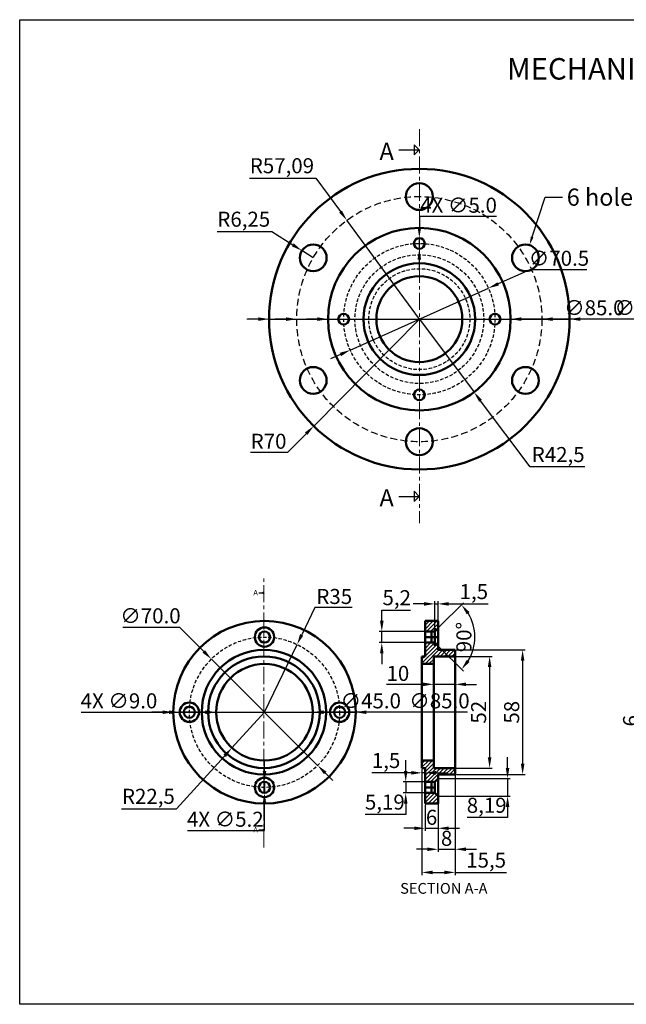
# Model space of a CAD drawing. Units: millimetres. Extents: x -42 to 606, y -195 to 264.
# Tile 1 of 3: x -42 to 240, y -195 to 264. Entities that reach past the tile are written whole.
import ezdxf
from ezdxf import colors
from ezdxf.entities.mleader import LeaderData, LeaderLine
from ezdxf.math import Vec2, Vec3

# ---------------------------------------------------------------- set-up
doc = ezdxf.new("R2010")
doc.units = ezdxf.units.MM
doc.header["$LTSCALE"] = 0.5
doc.linetypes.add('CENTER', pattern=[50.8, 31.75, -6.35, 6.35, -6.35])
doc.linetypes.add('HIDDEN', pattern=[9.525, 6.35, -3.175])
for name, color, linetype, lineweight in [('M-CNTR', 1, 'CENTER', 18), ('M-DIMS', 2, 'Continuous', 25), ('M-HATC', 8, 'Continuous', 18), ('M-HIDN', 4, 'HIDDEN', 25), ('M-OUTL', 7, 'Continuous', 50), ('M-SYMB', 3, 'Continuous', 25), ('M-TEXT', 3, 'Continuous', 25), ('M-TTLB', 7, 'Continuous', 25)]:
    doc.layers.add(name, color=color, linetype=linetype, lineweight=lineweight)
doc.styles.get("Standard").update_dxf_attribs({"font": 'arial.ttf'})
doc.dimstyles.new('ISO-25', dxfattribs={"dimtxt": 7, "dimasz": 5, "dimexe": 1.25, "dimexo": 0.625, "dimtad": 1, "dimtoh": 1, "dimtxsty": 'Standard', "dimcen": 2.5, "dimadec": 0, "dimazin": 0, "dimtfac": 1, "dimtmove": 0, "dimatfit": 3, "dimfxl": 1, "dimarcsym": 0})

# ---------------------------------------------------------------- blocks, each defined once
blk = doc.blocks.new('*D18')
at = {"layer": 'Defpoints', "color": 0, "ltscale": 0.5, "transparency": 16777216}
for p in [(88.97, 156.13), (94.25, 152.78)]:
    blk.add_point(p, dxfattribs=at)
at = {"layer": 'M-DIMS', "color": 0, "lineweight": -2, "ltscale": 0.5, "transparency": 16777216}
for p, q in [((49.45, 165.02), (75.01, 165.02)), ((75.01, 165.02), (84.76, 158.82)), ((94.25, 152.78), (88.97, 156.13))]:
    blk.add_line(p, q, dxfattribs=at)
at = {"layer": 'M-DIMS', "color": 0, "ltscale": 0.5, "transparency": 16777216}
blk.add_solid([(85.2, 159.52), (84.31, 158.11), (88.97, 156.13)], dxfattribs=at)
at = {"layer": 'M-DIMS', "color": 0, "ltscale": 0.5, "transparency": 16777216, "insert": (61.91, 169.85), "char_height": 7, "attachment_point": 5}
blk.add_mtext('R6,25', dxfattribs=at)
blk = doc.blocks.new('*D19')
at = {"layer": 'Defpoints', "color": 0, "ltscale": 0.5, "transparency": 16777216}
for p in [(143.69, 124.23), (94.49, 74.44)]:
    blk.add_point(p, dxfattribs=at)
at = {"layer": 'M-DIMS', "color": 0, "lineweight": -2, "ltscale": 0.5, "transparency": 16777216}
for p, q in [((143.69, 124.23), (94.49, 74.44)), ((82.43, 62.24), (90.97, 70.88)), ((65.11, 62.24), (82.43, 62.24))]:
    blk.add_line(p, q, dxfattribs=at)
at = {"layer": 'M-DIMS', "color": 0, "ltscale": 0.5, "transparency": 16777216}
blk.add_solid([(90.38, 71.47), (91.56, 70.3), (94.49, 74.44)], dxfattribs=at)
at = {"layer": 'M-DIMS', "color": 0, "ltscale": 0.5, "transparency": 16777216, "insert": (73.46, 66.44), "char_height": 7, "attachment_point": 5}
blk.add_mtext('R70', dxfattribs=at)
blk = doc.blocks.new('*D20')
at = {"layer": 'Defpoints', "color": 0, "ltscale": 0.5, "transparency": 16777216}
for p in [(143.69, 124.23), (169.18, 90.22)]:
    blk.add_point(p, dxfattribs=at)
at = {"layer": 'M-DIMS', "color": 0, "lineweight": -2, "ltscale": 0.5, "transparency": 16777216}
for p, q in [((143.69, 124.23), (169.18, 90.22)), ((195.26, 55.43), (172.18, 86.22)), ((220.82, 55.43), (195.26, 55.43))]:
    blk.add_line(p, q, dxfattribs=at)
at = {"layer": 'M-DIMS', "color": 0, "ltscale": 0.5, "transparency": 16777216}
blk.add_solid([(172.85, 86.72), (171.51, 85.72), (169.18, 90.22)], dxfattribs=at)
at = {"layer": 'M-DIMS', "color": 0, "ltscale": 0.5, "transparency": 16777216, "insert": (208.36, 60.26), "char_height": 7, "attachment_point": 5}
blk.add_mtext('R42,5', dxfattribs=at)
blk = doc.blocks.new('*D21')
at = {"layer": 'Defpoints', "color": 0, "ltscale": 0.5, "transparency": 16777216}
for p in [(109.92, 170.26), (143.69, 124.23)]:
    blk.add_point(p, dxfattribs=at)
at = {"layer": 'M-DIMS', "color": 0, "lineweight": -2, "ltscale": 0.5, "transparency": 16777216}
for p, q in [((64.53, 189.93), (95.49, 189.93)), ((95.49, 189.93), (106.96, 174.29)), ((143.69, 124.23), (109.92, 170.26))]:
    blk.add_line(p, q, dxfattribs=at)
at = {"layer": 'M-DIMS', "color": 0, "ltscale": 0.5, "transparency": 16777216}
blk.add_solid([(107.63, 174.78), (106.29, 173.8), (109.92, 170.26)], dxfattribs=at)
at = {"layer": 'M-DIMS', "color": 0, "ltscale": 0.5, "transparency": 16777216, "insert": (79.69, 194.76), "char_height": 7, "attachment_point": 5}
blk.add_mtext('R57,09', dxfattribs=at)
blk = doc.blocks.new('*D23')
at = {"layer": 'Defpoints', "color": 0, "ltscale": 0.5, "transparency": 16777216}
for p in [(255.34, -59.83), (247.18, -65.83), (255.34, -65.83)]:
    blk.add_point(p, dxfattribs=at)
at = {"layer": 'M-DIMS', "color": 0, "lineweight": -2, "ltscale": 0.5, "transparency": 16777216}
for p, q in [((247.18, -54.83), (247.18, -49.83)), ((254.71, -59.83), (245.93, -59.83)), ((247.18, -59.83), (247.18, -65.83)), ((254.71, -65.83), (245.93, -65.83)), ((247.18, -70.83), (247.18, -75.83))]:
    blk.add_line(p, q, dxfattribs=at)
at = {"layer": 'M-DIMS', "color": 0, "ltscale": 0.5, "transparency": 16777216}
for points in [[(246.34, -54.83), (248.01, -54.83), (247.18, -59.83)], [(246.34, -70.83), (248.01, -70.83), (247.18, -65.83)]]:
    blk.add_solid(points, dxfattribs=at)
at = {"layer": 'M-DIMS', "color": 0, "ltscale": 0.5, "transparency": 16777216, "insert": (242.98, -62.83), "char_height": 7, "attachment_point": 5, "rotation": 90}
blk.add_mtext('6', dxfattribs=at)
blk = doc.blocks.new('*D51')
at = {"layer": 'Defpoints', "color": 0, "ltscale": 0.5, "transparency": 16777216}
for p in [(160.39, -32.83), (160.39, -84.83), (176.42, -84.83)]:
    blk.add_point(p, dxfattribs=at)
at = {"layer": 'M-DIMS', "color": 0, "lineweight": -2, "ltscale": 0.5, "transparency": 16777216}
for p, q in [((161.01, -32.83), (177.67, -32.83)), ((176.42, -37.83), (176.42, -79.83)), ((161.01, -84.83), (177.67, -84.83))]:
    blk.add_line(p, q, dxfattribs=at)
at = {"layer": 'M-DIMS', "color": 0, "ltscale": 0.5, "transparency": 16777216}
for points in [[(175.58, -37.83), (177.25, -37.83), (176.42, -32.83)], [(175.58, -79.83), (177.25, -79.83), (176.42, -84.83)]]:
    blk.add_solid(points, dxfattribs=at)
at = {"layer": 'M-DIMS', "color": 0, "ltscale": 0.5, "transparency": 16777216, "insert": (172.22, -58.83), "char_height": 7, "attachment_point": 5, "rotation": 90}
blk.add_mtext('52', dxfattribs=at)
blk = doc.blocks.new('*D52')
at = {"layer": 'Defpoints', "color": 0, "ltscale": 0.5, "transparency": 16777216}
for p in [(160.39, -29.83), (160.39, -87.83), (191.8, -87.83)]:
    blk.add_point(p, dxfattribs=at)
at = {"layer": 'M-DIMS', "color": 0, "lineweight": -2, "ltscale": 0.5, "transparency": 16777216}
for p, q in [((161.01, -29.83), (193.05, -29.83)), ((191.8, -34.83), (191.8, -82.83)), ((161.01, -87.83), (193.05, -87.83))]:
    blk.add_line(p, q, dxfattribs=at)
at = {"layer": 'M-DIMS', "color": 0, "ltscale": 0.5, "transparency": 16777216}
for points in [[(190.97, -34.83), (192.63, -34.83), (191.8, -29.83)], [(190.97, -82.83), (192.63, -82.83), (191.8, -87.83)]]:
    blk.add_solid(points, dxfattribs=at)
at = {"layer": 'M-DIMS', "color": 0, "ltscale": 0.5, "transparency": 16777216, "insert": (187.6, -58.83), "char_height": 7, "attachment_point": 5, "rotation": 90}
blk.add_mtext('58', dxfattribs=at)
blk = doc.blocks.new('*D53')
at = {"layer": 'Defpoints', "color": 0, "ltscale": 0.5, "transparency": 16777216}
for p in [(152.39, -8.38), (150.89, -19.73), (152.39, -19.73)]:
    blk.add_point(p, dxfattribs=at)
at = {"layer": 'M-DIMS', "color": 0, "lineweight": -2, "ltscale": 0.5, "transparency": 16777216}
for p, q in [((145.89, -8.38), (140.89, -8.38)), ((150.89, -19.1), (150.89, -7.13)), ((150.89, -8.38), (152.39, -8.38)), ((152.39, -19.1), (152.39, -7.13)), ((157.39, -8.38), (175.78, -8.38))]:
    blk.add_line(p, q, dxfattribs=at)
at = {"layer": 'M-DIMS', "color": 0, "ltscale": 0.5, "transparency": 16777216}
for points in [[(145.89, -7.55), (145.89, -9.22), (150.89, -8.38)], [(157.39, -7.55), (157.39, -9.22), (152.39, -8.38)]]:
    blk.add_solid(points, dxfattribs=at)
at = {"layer": 'M-DIMS', "color": 0, "ltscale": 0.5, "transparency": 16777216, "insert": (169.08, -3.55), "char_height": 7, "attachment_point": 5}
blk.add_mtext('1,5', dxfattribs=at)
blk = doc.blocks.new('*D54')
at = {"layer": 'Defpoints', "color": 0, "ltscale": 0.5, "transparency": 16777216}
for p in [(146.39, -21.23), (126.2, -26.43), (146.39, -26.43)]:
    blk.add_point(p, dxfattribs=at)
at = {"layer": 'M-DIMS', "color": 0, "lineweight": -2, "ltscale": 0.5, "transparency": 16777216}
for p, q in [((126.2, -16.23), (126.2, -11.23)), ((126.2, -11.23), (139.5, -11.23)), ((145.76, -21.23), (124.95, -21.23)), ((126.2, -26.43), (126.2, -21.23)), ((145.76, -26.43), (124.95, -26.43)), ((126.2, -31.43), (126.2, -36.43))]:
    blk.add_line(p, q, dxfattribs=at)
at = {"layer": 'M-DIMS', "color": 0, "ltscale": 0.5, "transparency": 16777216}
for points in [[(125.37, -16.23), (127.03, -16.23), (126.2, -21.23)], [(125.37, -31.43), (127.03, -31.43), (126.2, -26.43)]]:
    blk.add_solid(points, dxfattribs=at)
at = {"layer": 'M-DIMS', "color": 0, "ltscale": 0.5, "transparency": 16777216, "insert": (133.16, -6.39), "char_height": 7, "attachment_point": 5}
blk.add_mtext('5,2', dxfattribs=at)
blk = doc.blocks.new('*D55')
at = {"layer": 'Defpoints', "color": 0, "ltscale": 0.5, "transparency": 16777216}
for p in [(160.39, -45.84), (150.39, -46.83), (160.39, -46.83)]:
    blk.add_point(p, dxfattribs=at)
at = {"layer": 'M-DIMS', "color": 0, "lineweight": -2, "ltscale": 0.5, "transparency": 16777216}
for p, q in [((145.39, -45.84), (128.4, -45.84)), ((150.39, -46.2), (150.39, -44.59)), ((160.39, -45.84), (150.39, -45.84)), ((160.39, -46.2), (160.39, -44.59)), ((165.39, -45.84), (170.39, -45.84))]:
    blk.add_line(p, q, dxfattribs=at)
at = {"layer": 'M-DIMS', "color": 0, "ltscale": 0.5, "transparency": 16777216}
for points in [[(145.39, -45.01), (145.39, -46.67), (150.39, -45.84)], [(165.39, -45.01), (165.39, -46.67), (160.39, -45.84)]]:
    blk.add_solid(points, dxfattribs=at)
at = {"layer": 'M-DIMS', "color": 0, "ltscale": 0.5, "transparency": 16777216, "insert": (133.7, -41.64), "char_height": 7, "attachment_point": 5}
blk.add_mtext('10', dxfattribs=at)
blk = doc.blocks.new('*D56')
at = {"layer": 'Defpoints', "color": 0, "ltscale": 0.5, "transparency": 16777216}
for p in [(144.89, -84.83), (144.89, -87.05), (146.39, -84.83)]:
    blk.add_point(p, dxfattribs=at)
at = {"layer": 'M-DIMS', "color": 0, "lineweight": -2, "ltscale": 0.5, "transparency": 16777216}
for p, q in [((139.89, -87.05), (121.5, -87.05)), ((144.89, -85.45), (144.89, -88.3)), ((146.39, -87.05), (144.89, -87.05)), ((146.39, -85.45), (146.39, -88.3)), ((151.39, -87.05), (156.39, -87.05))]:
    blk.add_line(p, q, dxfattribs=at)
at = {"layer": 'M-DIMS', "color": 0, "ltscale": 0.5, "transparency": 16777216}
for points in [[(139.89, -86.22), (139.89, -87.89), (144.89, -87.05)], [(151.39, -86.22), (151.39, -87.89), (146.39, -87.05)]]:
    blk.add_solid(points, dxfattribs=at)
at = {"layer": 'M-DIMS', "color": 0, "ltscale": 0.5, "transparency": 16777216, "insert": (128.2, -82.22), "char_height": 7, "attachment_point": 5}
blk.add_mtext('1,5', dxfattribs=at)
blk = doc.blocks.new('*D57')
at = {"layer": 'Defpoints', "color": 0, "ltscale": 0.5, "transparency": 16777216}
for p in [(150.89, -21.24), (152.39, -19.74), (150.89, -26.43), (152.39, -27.93), (168.83, -29.33)]:
    blk.add_point(p, dxfattribs=at)
at = {"layer": 'M-DIMS', "color": 0, "lineweight": -2, "ltscale": 0.5, "transparency": 16777216}
for p, q in [((152.83, -19.29), (164.21, -7.91)), ((152.83, -28.37), (164.21, -39.75))]:
    blk.add_line(p, q, dxfattribs=at)
blk.add_arc((148.29, -23.83), 21.26, 328.507, 31.493, dxfattribs=at)
at = {"layer": 'M-DIMS', "color": 0, "ltscale": 0.5, "transparency": 16777216}
for points in [[(165.77, -13.24), (167.08, -12.21), (163.33, -8.8)], [(167.08, -35.45), (165.77, -34.42), (163.33, -38.86)]]:
    blk.add_solid(points, dxfattribs=at)
at = {"layer": 'M-DIMS', "color": 0, "ltscale": 0.5, "transparency": 16777216, "insert": (165.35, -23.83), "char_height": 7, "attachment_point": 5, "rotation": 90}
blk.add_mtext('90°', dxfattribs=at)
blk = doc.blocks.new('*D58')
at = {"layer": 'Defpoints', "color": 0, "ltscale": 0.5, "transparency": 16777216}
for p in [(146.39, -101.33), (152.39, -101.33), (152.39, -112.87)]:
    blk.add_point(p, dxfattribs=at)
at = {"layer": 'M-DIMS', "color": 0, "lineweight": -2, "ltscale": 0.5, "transparency": 16777216}
for p, q in [((146.39, -101.95), (146.39, -114.12)), ((152.39, -101.95), (152.39, -114.12)), ((141.39, -112.87), (136.39, -112.87)), ((146.39, -112.87), (152.39, -112.87)), ((157.39, -112.87), (162.39, -112.87))]:
    blk.add_line(p, q, dxfattribs=at)
at = {"layer": 'M-DIMS', "color": 0, "ltscale": 0.5, "transparency": 16777216}
for points in [[(141.39, -112.04), (141.39, -113.7), (146.39, -112.87)], [(157.39, -112.04), (157.39, -113.7), (152.39, -112.87)]]:
    blk.add_solid(points, dxfattribs=at)
at = {"layer": 'M-DIMS', "color": 0, "ltscale": 0.5, "transparency": 16777216, "insert": (149.39, -108.67), "char_height": 7, "attachment_point": 5}
blk.add_mtext('6', dxfattribs=at)
blk = doc.blocks.new('*D59')
at = {"layer": 'Defpoints', "color": 0, "ltscale": 0.5, "transparency": 16777216}
for p in [(152.39, -87.83), (160.39, -87.83), (160.39, -122.64)]:
    blk.add_point(p, dxfattribs=at)
at = {"layer": 'M-DIMS', "color": 0, "lineweight": -2, "ltscale": 0.5, "transparency": 16777216}
for p, q in [((152.39, -88.45), (152.39, -123.89)), ((160.39, -88.45), (160.39, -123.89)), ((147.39, -122.64), (142.39, -122.64)), ((152.39, -122.64), (160.39, -122.64)), ((165.39, -122.64), (170.39, -122.64))]:
    blk.add_line(p, q, dxfattribs=at)
at = {"layer": 'M-DIMS', "color": 0, "ltscale": 0.5, "transparency": 16777216}
for points in [[(147.39, -121.81), (147.39, -123.47), (152.39, -122.64)], [(165.39, -121.81), (165.39, -123.47), (160.39, -122.64)]]:
    blk.add_solid(points, dxfattribs=at)
at = {"layer": 'M-DIMS', "color": 0, "ltscale": 0.5, "transparency": 16777216, "insert": (156.39, -118.44), "char_height": 7, "attachment_point": 5}
blk.add_mtext('8', dxfattribs=at)
blk = doc.blocks.new('*D60')
at = {"layer": 'Defpoints', "color": 0, "ltscale": 0.5, "transparency": 16777216}
for p in [(144.89, -84.83), (160.39, -84.83), (160.39, -133.42)]:
    blk.add_point(p, dxfattribs=at)
at = {"layer": 'M-DIMS', "color": 0, "lineweight": -2, "ltscale": 0.5, "transparency": 16777216}
for p, q in [((144.89, -85.45), (144.89, -134.67)), ((160.39, -85.45), (160.39, -134.67)), ((149.89, -133.42), (155.39, -133.42)), ((160.39, -133.42), (184.22, -133.42))]:
    blk.add_line(p, q, dxfattribs=at)
at = {"layer": 'M-DIMS', "color": 0, "ltscale": 0.5, "transparency": 16777216}
for points in [[(149.89, -132.59), (149.89, -134.26), (144.89, -133.42)], [(155.39, -132.59), (155.39, -134.26), (160.39, -133.42)]]:
    blk.add_solid(points, dxfattribs=at)
at = {"layer": 'M-DIMS', "color": 0, "ltscale": 0.5, "transparency": 16777216, "insert": (174.8, -128.59), "char_height": 7, "attachment_point": 5}
blk.add_mtext('15,5', dxfattribs=at)
blk = doc.blocks.new('*D61')
at = {"layer": 'Defpoints', "color": 0, "ltscale": 0.5, "transparency": 16777216}
for p in [(146.39, -91.23), (137.35, -96.41), (146.39, -96.41)]:
    blk.add_point(p, dxfattribs=at)
at = {"layer": 'M-DIMS', "color": 0, "lineweight": -2, "ltscale": 0.5, "transparency": 16777216}
for p, q in [((137.35, -86.23), (137.35, -81.23)), ((145.76, -91.23), (136.1, -91.23)), ((137.35, -91.23), (137.35, -96.41)), ((145.76, -96.41), (136.1, -96.41)), ((137.35, -101.41), (137.35, -106.41)), ((137.35, -106.41), (118.53, -106.41))]:
    blk.add_line(p, q, dxfattribs=at)
at = {"layer": 'M-DIMS', "color": 0, "ltscale": 0.5, "transparency": 16777216}
for points in [[(136.51, -86.23), (138.18, -86.23), (137.35, -91.23)], [(136.51, -101.41), (138.18, -101.41), (137.35, -96.41)]]:
    blk.add_solid(points, dxfattribs=at)
at = {"layer": 'M-DIMS', "color": 0, "ltscale": 0.5, "transparency": 16777216, "insert": (127.62, -101.58), "char_height": 7, "attachment_point": 5}
blk.add_mtext('5,19', dxfattribs=at)
blk = doc.blocks.new('*D62')
at = {"layer": 'Defpoints', "color": 0, "ltscale": 0.5, "transparency": 16777216}
for p in [(152.39, -89.73), (152.39, -97.91), (184.79, -97.91)]:
    blk.add_point(p, dxfattribs=at)
at = {"layer": 'M-DIMS', "color": 0, "lineweight": -2, "ltscale": 0.5, "transparency": 16777216}
for p, q in [((184.79, -84.73), (184.79, -79.73)), ((153.01, -89.73), (186.04, -89.73)), ((184.79, -89.73), (184.79, -97.91)), ((153.01, -97.91), (186.04, -97.91)), ((184.79, -102.91), (184.79, -107.91)), ((184.79, -107.91), (165.96, -107.91))]:
    blk.add_line(p, q, dxfattribs=at)
at = {"layer": 'M-DIMS', "color": 0, "ltscale": 0.5, "transparency": 16777216}
for points in [[(183.95, -84.73), (185.62, -84.73), (184.79, -89.73)], [(183.95, -102.91), (185.62, -102.91), (184.79, -97.91)]]:
    blk.add_solid(points, dxfattribs=at)
at = {"layer": 'M-DIMS', "color": 0, "ltscale": 0.5, "transparency": 16777216, "insert": (175.06, -103.08), "char_height": 7, "attachment_point": 5}
blk.add_mtext('8,19', dxfattribs=at)
blk = doc.blocks.new('*D63')
at = {"layer": 'Defpoints', "color": 0, "ltscale": 0.5, "transparency": 16777216}
for p in [(71.56, -58.83), (56.39, -75.44)]:
    blk.add_point(p, dxfattribs=at)
at = {"layer": 'M-DIMS', "color": 0, "lineweight": -2, "ltscale": 0.5, "transparency": 16777216}
for p, q in [((71.56, -58.83), (56.39, -75.44)), ((30.57, -103.74), (53.02, -79.14)), ((5.01, -103.74), (30.57, -103.74))]:
    blk.add_line(p, q, dxfattribs=at)
at = {"layer": 'M-DIMS', "color": 0, "ltscale": 0.5, "transparency": 16777216}
blk.add_solid([(52.41, -78.58), (53.64, -79.7), (56.39, -75.44)], dxfattribs=at)
at = {"layer": 'M-DIMS', "color": 0, "ltscale": 0.5, "transparency": 16777216, "insert": (17.48, -98.9), "char_height": 7, "attachment_point": 5}
blk.add_mtext('R22,5', dxfattribs=at)
blk = doc.blocks.new('*D64')
at = {"layer": 'Defpoints', "color": 0, "ltscale": 0.5, "transparency": 16777216}
for p in [(86.74, -27.29), (71.56, -58.83)]:
    blk.add_point(p, dxfattribs=at)
at = {"layer": 'M-DIMS', "color": 0, "lineweight": -2, "ltscale": 0.5, "transparency": 16777216}
for p, q in [((95.04, -10.03), (88.9, -22.78)), ((112.44, -10.03), (95.04, -10.03)), ((71.56, -58.83), (86.74, -27.29))]:
    blk.add_line(p, q, dxfattribs=at)
at = {"layer": 'M-DIMS', "color": 0, "ltscale": 0.5, "transparency": 16777216}
blk.add_solid([(88.15, -22.42), (89.65, -23.14), (86.74, -27.29)], dxfattribs=at)
at = {"layer": 'M-DIMS', "color": 0, "ltscale": 0.5, "transparency": 16777216, "insert": (104.05, -5.83), "char_height": 7, "attachment_point": 5}
blk.add_mtext('R35', dxfattribs=at)
blk = doc.blocks.new('SECTION-ARROW')
at = {"ltscale": 0.5}
for p, q in [((0, 0.39), (2.47, 0.39)), ((2.47, 0.39), (2.07, 0.78)), ((2.07, 0.78), (2.07, 0)), ((2.47, 0.39), (2.07, 0))]:
    blk.add_line(p, q, dxfattribs=at)
blk = doc.blocks.new('SECTION-ARROW-LG')
at = {"ltscale": 0.5}
for p, q in [((9.52, 2.39), (7.13, 4.78)), ((7.13, 4.78), (7.13, 0)), ((0, 2.39), (9.52, 2.39)), ((9.52, 2.39), (7.13, 0))]:
    blk.add_line(p, q, dxfattribs=at)
blk = doc.blocks.new('*D68')
at = {"layer": 'Defpoints', "color": 0, "ltscale": 0.5, "transparency": 16777216}
for p in [(73.69, 124.23), (213.69, 124.23)]:
    blk.add_point(p, dxfattribs=at)
at = {"layer": 'M-DIMS', "color": 0, "lineweight": -2, "ltscale": 0.5, "transparency": 16777216}
for p, q in [((68.69, 124.23), (63.69, 124.23)), ((73.69, 124.23), (213.69, 124.23)), ((255.69, 124.23), (218.69, 124.23)), ((287.53, 124.23), (255.69, 124.23))]:
    blk.add_line(p, q, dxfattribs=at)
at = {"layer": 'M-DIMS', "color": 0, "ltscale": 0.5, "transparency": 16777216}
for points in [[(68.69, 125.06), (68.69, 123.4), (73.69, 124.23)], [(218.69, 125.06), (218.69, 123.4), (213.69, 124.23)]]:
    blk.add_solid(points, dxfattribs=at)
at = {"layer": 'M-DIMS', "color": 0, "ltscale": 0.5, "transparency": 16777216, "insert": (271.92, 128.62), "char_height": 7, "attachment_point": 5}
blk.add_mtext('∅140.0', dxfattribs=at)
blk = doc.blocks.new('*D69')
at = {"layer": 'Defpoints', "color": 0, "ltscale": 0.5, "transparency": 16777216}
for p in [(86.6, 124.23), (200.78, 124.23)]:
    blk.add_point(p, dxfattribs=at)
at = {"layer": 'M-DIMS', "color": 0, "lineweight": -2, "ltscale": 0.5, "transparency": 16777216}
for p, q in [((81.6, 124.23), (76.6, 124.23)), ((86.6, 124.23), (200.78, 124.23)), ((235.03, 124.23), (205.78, 124.23)), ((272.35, 124.23), (235.03, 124.23))]:
    blk.add_line(p, q, dxfattribs=at)
at = {"layer": 'M-DIMS', "color": 0, "ltscale": 0.5, "transparency": 16777216}
for points in [[(81.6, 125.06), (81.6, 123.4), (86.6, 124.23)], [(205.78, 125.06), (205.78, 123.4), (200.78, 124.23)]]:
    blk.add_solid(points, dxfattribs=at)
at = {"layer": 'M-DIMS', "color": 0, "ltscale": 0.5, "transparency": 16777216, "insert": (254, 128.62), "char_height": 7, "attachment_point": 5}
blk.add_mtext('∅114.18', dxfattribs=at)
blk = doc.blocks.new('*D70')
at = {"layer": 'Defpoints', "color": 0, "ltscale": 0.5, "transparency": 16777216}
for p in [(101.19, 124.23), (186.19, 124.23)]:
    blk.add_point(p, dxfattribs=at)
at = {"layer": 'M-DIMS', "color": 0, "lineweight": -2, "ltscale": 0.5, "transparency": 16777216}
for p, q in [((96.19, 124.23), (91.19, 124.23)), ((101.19, 124.23), (186.19, 124.23)), ((211.69, 124.23), (191.19, 124.23)), ((238.09, 124.23), (211.69, 124.23))]:
    blk.add_line(p, q, dxfattribs=at)
at = {"layer": 'M-DIMS', "color": 0, "ltscale": 0.5, "transparency": 16777216}
for points in [[(96.19, 125.06), (96.19, 123.4), (101.19, 124.23)], [(191.19, 125.06), (191.19, 123.4), (186.19, 124.23)]]:
    blk.add_solid(points, dxfattribs=at)
at = {"layer": 'M-DIMS', "color": 0, "ltscale": 0.5, "transparency": 16777216, "insert": (225.2, 128.62), "char_height": 7, "attachment_point": 5}
blk.add_mtext('∅85.0', dxfattribs=at)
blk = doc.blocks.new('*D71')
at = {"layer": 'Defpoints', "color": 0, "ltscale": 0.5, "transparency": 16777216}
for p in [(143.69, 161.98), (143.69, 156.98)]:
    blk.add_point(p, dxfattribs=at)
at = {"layer": 'M-DIMS', "color": 0, "lineweight": -2, "ltscale": 0.5, "transparency": 16777216}
for p, q in [((143.7, 171.98), (143.69, 166.98)), ((179.61, 171.98), (143.7, 171.98)), ((143.69, 156.98), (143.69, 161.98)), ((143.68, 151.98), (143.68, 146.98))]:
    blk.add_line(p, q, dxfattribs=at)
at = {"layer": 'M-DIMS', "color": 0, "ltscale": 0.5, "transparency": 16777216}
for points in [[(142.86, 166.98), (144.53, 166.98), (143.69, 161.98)], [(142.85, 151.98), (144.51, 151.98), (143.69, 156.98)]]:
    blk.add_solid(points, dxfattribs=at)
at = {"layer": 'M-DIMS', "color": 0, "ltscale": 0.5, "transparency": 16777216, "insert": (161.97, 176.38), "char_height": 7, "attachment_point": 5}
blk.add_mtext('4X ∅5.0', dxfattribs=at)
blk = doc.blocks.new('*D72')
at = {"layer": 'Defpoints', "color": 0, "ltscale": 0.5, "transparency": 16777216}
for p in [(175.86, 138.63), (111.51, 109.84)]:
    blk.add_point(p, dxfattribs=at)
at = {"layer": 'M-DIMS', "color": 0, "lineweight": -2, "ltscale": 0.5, "transparency": 16777216}
for p, q in [((195.17, 147.26), (180.43, 140.67)), ((221.65, 147.26), (195.17, 147.26)), ((111.51, 109.84), (175.86, 138.63)), ((106.95, 107.79), (102.38, 105.75))]:
    blk.add_line(p, q, dxfattribs=at)
at = {"layer": 'M-DIMS', "color": 0, "ltscale": 0.5, "transparency": 16777216}
for points in [[(180.09, 141.43), (180.77, 139.91), (175.86, 138.63)], [(106.61, 108.55), (107.29, 107.03), (111.51, 109.84)]]:
    blk.add_solid(points, dxfattribs=at)
at = {"layer": 'M-DIMS', "color": 0, "ltscale": 0.5, "transparency": 16777216, "insert": (208.72, 151.66), "char_height": 7, "attachment_point": 5}
blk.add_mtext('∅70.5', dxfattribs=at)
blk = doc.blocks.new('*D74')
at = {"layer": 'Defpoints', "color": 0, "ltscale": 0.5, "transparency": 16777216}
for p in [(29.06, -58.83), (114.06, -58.82)]:
    blk.add_point(p, dxfattribs=at)
at = {"layer": 'M-DIMS', "color": 0, "lineweight": -2, "ltscale": 0.5, "transparency": 16777216}
for p, q in [((24.06, -58.83), (19.06, -58.83)), ((29.06, -58.83), (114.06, -58.82)), ((139.56, -58.82), (119.06, -58.82)), ((165.96, -58.82), (139.56, -58.82))]:
    blk.add_line(p, q, dxfattribs=at)
at = {"layer": 'M-DIMS', "color": 0, "ltscale": 0.5, "transparency": 16777216}
for points in [[(24.06, -57.99), (24.06, -59.66), (29.06, -58.83)], [(119.06, -57.99), (119.06, -59.66), (114.06, -58.82)]]:
    blk.add_solid(points, dxfattribs=at)
at = {"layer": 'M-DIMS', "color": 0, "ltscale": 0.5, "transparency": 16777216, "insert": (153.07, -54.43), "char_height": 7, "attachment_point": 5}
blk.add_mtext('∅85.0', dxfattribs=at)
blk = doc.blocks.new('*D75')
at = {"layer": 'Defpoints', "color": 0, "ltscale": 0.5, "transparency": 16777216}
for p in [(46.81, -34.07), (96.31, -83.58)]:
    blk.add_point(p, dxfattribs=at)
at = {"layer": 'M-DIMS', "color": 0, "lineweight": -2, "ltscale": 0.5, "transparency": 16777216}
for p, q in [((5.57, -19.22), (31.97, -19.22)), ((31.97, -19.22), (43.28, -30.54)), ((96.31, -83.58), (46.81, -34.07)), ((99.84, -87.11), (103.38, -90.65))]:
    blk.add_line(p, q, dxfattribs=at)
at = {"layer": 'M-DIMS', "color": 0, "ltscale": 0.5, "transparency": 16777216}
for points in [[(43.87, -29.95), (42.69, -31.13), (46.81, -34.07)], [(100.43, -86.52), (99.25, -87.7), (96.31, -83.58)]]:
    blk.add_solid(points, dxfattribs=at)
at = {"layer": 'M-DIMS', "color": 0, "ltscale": 0.5, "transparency": 16777216, "insert": (18.45, -14.83), "char_height": 7, "attachment_point": 5}
blk.add_mtext('∅70.0', dxfattribs=at)
blk = doc.blocks.new('*D76')
at = {"layer": 'Defpoints', "color": 0, "ltscale": 0.5, "transparency": 16777216}
for p in [(49.06, -58.83), (94.06, -58.83)]:
    blk.add_point(p, dxfattribs=at)
at = {"layer": 'M-DIMS', "color": 0, "lineweight": -2, "ltscale": 0.5, "transparency": 16777216}
for p, q in [((44.06, -58.83), (39.06, -58.83)), ((49.06, -58.83), (94.06, -58.83)), ((107.56, -58.82), (99.06, -58.83)), ((133.96, -58.82), (107.56, -58.82))]:
    blk.add_line(p, q, dxfattribs=at)
at = {"layer": 'M-DIMS', "color": 0, "ltscale": 0.5, "transparency": 16777216}
for points in [[(44.06, -57.99), (44.06, -59.66), (49.06, -58.83)], [(99.06, -57.99), (99.06, -59.66), (94.06, -58.83)]]:
    blk.add_solid(points, dxfattribs=at)
at = {"layer": 'M-DIMS', "color": 0, "ltscale": 0.5, "transparency": 16777216, "insert": (121.07, -54.43), "char_height": 7, "attachment_point": 5}
blk.add_mtext('∅45.0', dxfattribs=at)
blk = doc.blocks.new('*D77')
at = {"layer": 'Defpoints', "color": 0, "ltscale": 0.5, "transparency": 16777216}
for p in [(32.06, -58.83), (41.06, -58.83)]:
    blk.add_point(p, dxfattribs=at)
at = {"layer": 'M-DIMS', "color": 0, "lineweight": -2, "ltscale": 0.5, "transparency": 16777216}
for p, q in [((-13.85, -58.82), (22.06, -58.82)), ((22.06, -58.82), (27.06, -58.82)), ((41.06, -58.83), (32.06, -58.83)), ((46.06, -58.83), (51.06, -58.83))]:
    blk.add_line(p, q, dxfattribs=at)
at = {"layer": 'M-DIMS', "color": 0, "ltscale": 0.5, "transparency": 16777216}
for points in [[(27.06, -57.99), (27.06, -59.66), (32.06, -58.83)], [(46.06, -57.99), (46.06, -59.66), (41.06, -58.83)]]:
    blk.add_solid(points, dxfattribs=at)
at = {"layer": 'M-DIMS', "color": 0, "ltscale": 0.5, "transparency": 16777216, "insert": (3.79, -54.43), "char_height": 7, "attachment_point": 5}
blk.add_mtext('4X ∅9.0', dxfattribs=at)
blk = doc.blocks.new('*D78')
at = {"layer": 'Defpoints', "color": 0, "ltscale": 0.5, "transparency": 16777216}
for p in [(71.56, -91.23), (71.56, -96.43)]:
    blk.add_point(p, dxfattribs=at)
at = {"layer": 'M-DIMS', "color": 0, "lineweight": -2, "ltscale": 0.5, "transparency": 16777216}
for p, q in [((71.57, -86.23), (71.57, -81.23)), ((71.56, -91.23), (71.56, -96.43)), ((71.55, -113.96), (71.56, -101.43)), ((35.69, -113.96), (71.55, -113.96))]:
    blk.add_line(p, q, dxfattribs=at)
at = {"layer": 'M-DIMS', "color": 0, "ltscale": 0.5, "transparency": 16777216}
for points in [[(70.73, -86.22), (72.4, -86.23), (71.56, -91.23)], [(70.72, -101.42), (72.39, -101.43), (71.56, -96.43)]]:
    blk.add_solid(points, dxfattribs=at)
at = {"layer": 'M-DIMS', "color": 0, "ltscale": 0.5, "transparency": 16777216, "insert": (53.31, -109.57), "char_height": 7, "attachment_point": 5}
blk.add_mtext('4X ∅5.2', dxfattribs=at)

msp = doc.modelspace()

# ---------------------------------------------------------------- hatches: boundary and pattern name
at = {"layer": 'M-HATC', "ltscale": 0.5}
h = msp.add_hatch(dxfattribs=at)
h.set_pattern_fill('ANSI31', color=256, scale=0.4)
h.set_pattern_definition([(45, (152.1326, 0), (-0.898026, 0.898026), [])])
h.paths.add_polyline_path([(152.389, -16.325), (146.389, -16.325), (146.389, -21.237), (150.889, -21.237), (152.389, -19.737)])
h.paths.add_polyline_path([(160.389, -29.825), (152.389, -29.825), (152.389, -27.925), (150.889, -26.425), (146.389, -26.425), (146.389, -32.825), (144.889, -32.825), (144.889, -36.325), (150.389, -36.325), (150.389, -32.825), (160.389, -32.825)])
h.paths.add_polyline_path([(152.389, -97.914), (150.889, -96.414), (146.389, -96.414), (146.389, -101.325), (152.389, -101.325)])
h.paths.add_polyline_path([(150.389, -81.325), (144.889, -81.325), (144.889, -84.825), (146.389, -84.825), (146.389, -91.225), (150.889, -91.225), (152.389, -89.725), (152.389, -87.825), (160.389, -87.825), (160.389, -84.825), (150.389, -84.825)])

# ---------------------------------------------------------------- linework, layer by layer
at = {"layer": 'M-CNTR', "ltscale": 0.5}
for p, q in [((143.688, 212.644), (143.688, 29.208)), ((63.337, 124.23), (223.604, 124.23)), ((71.316, -121.894), (71.316, 4.622)), ((166.05, -58.825), (5.998, -58.825))]:
    msp.add_line(p, q, dxfattribs=at)
at = {"layer": 'M-HIDN'}
msp.add_circle((143.688, 124.23), 57.09, dxfattribs=at)
at = {"layer": 'M-HIDN', "ltscale": 0.5}
for centre, radius in [((143.688, 124.23), 35.25), ((143.688, 124.23), 30), ((143.688, 124.23), 23.5), ((71.561, -58.825), 35)]:
    msp.add_circle(centre, radius, dxfattribs=at)
at = {"layer": 'M-OUTL', "ltscale": 0.5}
for p, q in [((152.389, -16.325), (146.389, -16.325)), ((146.389, -16.325), (146.389, -32.825)), ((152.389, -29.825), (152.389, -16.325)), ((146.389, -21.237), (150.889, -21.237)), ((149.389, -23.825), (149.389, -21.225)), ((149.389, -21.225), (149.389, -26.425)), ((150.889, -19.725), (150.889, -27.925)), ((150.889, -21.237), (152.389, -19.737)), ((150.889, -21.237), (150.889, -26.425)), ((146.389, -23.825), (152.389, -23.825)), ((146.389, -23.825), (150.889, -23.825)), ((146.389, -26.425), (150.889, -26.425)), ((150.889, -26.425), (152.389, -27.925)), ((160.389, -29.825), (152.389, -29.825)), ((160.389, -29.825), (160.389, -87.825)), ((146.389, -32.825), (144.889, -32.825)), ((144.889, -32.825), (144.889, -84.825)), ((144.889, -36.325), (150.389, -36.325)), ((150.389, -84.825), (150.389, -32.825)), ((150.389, -32.825), (160.389, -32.825)), ((144.889, -81.325), (150.389, -81.325)), ((144.889, -84.825), (146.389, -84.825)), ((146.389, -84.825), (146.389, -101.325)), ((160.389, -84.825), (150.389, -84.825)), ((146.389, -91.225), (149.389, -91.225)), ((146.389, -91.225), (150.889, -91.225)), ((149.389, -96.414), (149.389, -91.225)), ((150.889, -91.225), (152.389, -89.725)), ((150.889, -96.414), (150.889, -91.225)), ((160.389, -87.825), (152.389, -87.825)), ((152.389, -87.825), (152.389, -101.325)), ((146.389, -93.825), (150.889, -93.825)), ((149.389, -93.825), (149.389, -96.414)), ((146.389, -96.414), (150.889, -96.414)), ((150.889, -96.414), (152.389, -97.914)), ((146.389, -101.325), (152.389, -101.325))]:
    msp.add_line(p, q, dxfattribs=at)
at = {"layer": 'M-OUTL'}
for centre, radius in [((143.688, 124.23), 70), ((143.688, 181.32), 6.25), ((94.246, 152.775), 6.25), ((193.129, 152.775), 6.25), ((94.246, 95.685), 6.25), ((193.129, 95.685), 6.25), ((143.688, 67.14), 6.25)]:
    msp.add_circle(centre, radius, dxfattribs=at)
at = {"layer": 'M-OUTL', "ltscale": 0.5}
for centre, radius in [((143.688, 124.23), 42.5), ((143.688, 159.48), 2.5), ((143.688, 124.23), 26), ((143.688, 124.23), 20), ((108.438, 124.23), 2.5), ((178.938, 124.23), 2.5), ((143.688, 88.98), 2.5), ((71.561, -58.825), 42.5), ((71.561, -23.825), 4.5), ((71.561, -23.825), 2.6), ((71.316, -58.825), 29), ((71.316, -58.825), 26), ((71.561, -58.825), 22.5), ((36.561, -58.825), 4.5), ((106.561, -58.825), 4.5), ((36.561, -58.825), 2.6), ((106.561, -58.825), 2.6), ((71.561, -93.825), 4.5), ((71.561, -93.825), 2.6)]:
    msp.add_circle(centre, radius, dxfattribs=at)
at = {"layer": 'M-TTLB', "ltscale": 0.5}
msp.add_lwpolyline([(-42.468, 263.673), (605.533, 263.673), (605.533, -194.845), (-42.468, -194.845)], close=True, dxfattribs=at)

# ---------------------------------------------------------------- block references
at = {"layer": 'M-SYMB'}
for name, p in [('SECTION-ARROW-LG', (134.165, 200.663)), ('SECTION-ARROW-LG', (134.165, 39.284)), ('SECTION-ARROW', (68.851, -3.618)), ('SECTION-ARROW', (68.851, -114.047))]:
    msp.add_blockref(name, p, dxfattribs=at)

# ---------------------------------------------------------------- texts
at = {"layer": 'M-TEXT', "insert": (156.416, 245.778), "char_height": 10, "width": 264.42118, "attachment_point": 1}
msp.add_mtext('\\pxqc;MECHANICAL FLANGE ASSEMBLY ', dxfattribs=at)
at = {"layer": 'M-TEXT', "ltscale": 0.5, "attachment_point": 1}
for s, width, heights, insert, char_height in [('A', 8, [2.244], (125.137, 206.399), 8), ('A', 8, [2.244], (125.137, 45.02), 8), ('A', 3.30931, [0], (66.389, -1.877), 2.5), ('A', 3.30931, [0], (66.389, -112.306), 2.5), ('SECTION A-A', 74.73507, [0], (134.748, -138.357), 5)]:
    msp.add_mtext_dynamic_manual_height_columns(s, width=width, gutter_width=12.5, heights=heights, dxfattribs=dict(at, insert=insert, char_height=char_height))

# ---------------------------------------------------------------- dimensions: what is measured, and where the dimension line sits
at = {"layer": 'M-DIMS', "ltscale": 0.5}
for center, mpoint, picture, middle in [((143.688, 124.23), (109.916, 170.26), '*D21', (79.693, 189.93)), ((94.246, 152.775), (88.974, 156.131), '*D18', (61.914, 165.019)), ((143.688, 124.23), (169.18, 90.224), '*D20', (208.357, 55.428)), ((71.561, -58.825), (86.735, -27.286), '*D64', (104.05, -10.033)), ((71.561, -58.825), (56.394, -75.444), '*D63', (17.48, -103.737))]:
    dim = msp.add_radius_dim(center=center, mpoint=mpoint, dimstyle='ISO-25', override={"dimclrd": 0, "dimclre": 0, "dimclrt": 0}, dxfattribs=at)
    dim.commit()
    dim.dimension.update_dxf_attribs({"geometry": picture, "text_midpoint": middle, "dimtype": 164})
for p1, p2, picture, middle in [((143.686, 156.98), (143.69, 161.98), '*D71', (161.967, 171.98)), ((41.061, -58.826), (32.061, -58.825), '*D77', (22.061, -58.824))]:
    dim = msp.add_diameter_dim_2p(p1=p1, p2=p2, text='4X <>', dimstyle='ISO-25', override={"dimdec": 1, "dimlfac": 1, "dimrnd": 0, "dimzin": 0, "dimdsep": 46, "dimlunit": 2}, dxfattribs=at)
    dim.commit()
    dim.dimension.update_dxf_attribs({"geometry": picture, "text_midpoint": middle, "dimtype": 163})
for p1, p2, override, picture, middle in [((111.511, 109.836), (175.865, 138.625), {"dimdec": 1, "dimlfac": 1, "dimrnd": 0, "dimzin": 0, "dimdsep": 46, "dimlunit": 2}, '*D72', (208.722, 147.262)), ((73.688, 124.231), (213.688, 124.23), {"dimdec": 1, "dimlfac": 1, "dimrnd": 0, "dimzin": 0, "dimdsep": 46, "dimlunit": 2}, '*D68', (255.688, 124.23)), ((86.598, 124.231), (200.778, 124.23), {"dimdec": 2, "dimlfac": 1, "dimrnd": 0, "dimzin": 0, "dimdsep": 46, "dimlunit": 2}, '*D69', (235.032, 124.23)), ((101.188, 124.231), (186.188, 124.23), {"dimdec": 1, "dimlfac": 1, "dimrnd": 0, "dimzin": 0, "dimdsep": 46, "dimlunit": 2}, '*D70', (211.688, 124.23)), ((96.308, -83.576), (46.815, -34.075), {"dimdec": 1, "dimlfac": 1, "dimrnd": 0, "dimzin": 0, "dimdsep": 46, "dimlunit": 2}, '*D75', (18.454, -19.224)), ((29.061, -58.826), (114.061, -58.825), {"dimdec": 1, "dimlfac": 1, "dimrnd": 0, "dimzin": 0, "dimdsep": 46, "dimlunit": 2}, '*D74', (139.561, -58.825)), ((49.061, -58.826), (94.061, -58.825), {"dimdec": 1, "dimlfac": 1, "dimrnd": 0, "dimzin": 0, "dimdsep": 46, "dimlunit": 2}, '*D76', (107.561, -58.825))]:
    dim = msp.add_diameter_dim_2p(p1=p1, p2=p2, dimstyle='ISO-25', override=override, dxfattribs=at)
    dim.commit()
    dim.dimension.update_dxf_attribs({"geometry": picture, "text_midpoint": middle, "dimtype": 163})
dim = msp.add_radius_dim(center=(143.688, 124.23), mpoint=(94.486, 74.439), dimstyle='ISO-25', override={"dimclrd": 0, "dimclre": 0, "dimclrt": 0}, dxfattribs=at)
dim.commit()
dim.dimension.update_dxf_attribs({"geometry": '*D19', "text_midpoint": (73.457, 66.44)})
for base, p1, p2, picture, middle in [((152.389, -8.385), (150.889, -19.725), (152.389, -19.725), '*D53', (169.083, -3.553)), ((144.889, -87.053), (146.389, -84.825), (144.889, -84.825), '*D56', (128.195, -82.221)), ((160.389, -133.424), (144.889, -84.825), (160.389, -84.825), '*D60', (174.802, -128.592)), ((160.389, -122.638), (152.389, -87.825), (160.389, -87.825), '*D59', (156.389, -118.439)), ((152.389, -112.869), (146.389, -101.325), (152.389, -101.325), '*D58', (149.389, -108.67))]:
    dim = msp.add_linear_dim(base=base, p1=p1, p2=p2, dimstyle='ISO-25', override={"dimclrd": 0, "dimclre": 0, "dimclrt": 0}, dxfattribs=at)
    dim.commit()
    dim.dimension.update_dxf_attribs({"geometry": picture, "text_midpoint": middle})
dim = msp.add_linear_dim(base=(126.201, -26.425), p1=(146.389, -21.225), p2=(146.389, -26.425), angle=90, dimstyle='ISO-25', override={"dimclrd": 0, "dimclre": 0, "dimclrt": 0}, dxfattribs=at)
dim.commit()
dim.dimension.update_dxf_attribs({"geometry": '*D54', "text_midpoint": (133.162, -11.225), "dimtype": 160})
dim = msp.add_angular_dim_2l(base=(168.83, -29.333), line1=((150.889, -26.425), (152.389, -27.925)), line2=((150.889, -21.237), (152.389, -19.737)), dimstyle='ISO-25', override={"dimclrd": 0, "dimclre": 0, "dimclrt": 0}, dxfattribs=at)
dim.commit()
dim.dimension.update_dxf_attribs({"geometry": '*D57', "text_midpoint": (165.355, -23.831)})
for base, p1, p2, picture, middle in [((191.799, -87.825), (160.389, -29.825), (160.389, -87.825), '*D52', (187.6, -58.825)), ((176.417, -84.825), (160.389, -32.825), (160.389, -84.825), '*D51', (172.218, -58.825)), ((247.175, -65.826), (255.339, -59.826), (255.339, -65.826), '*D23', (242.976, -62.826)), ((137.348, -96.414), (146.389, -91.225), (146.389, -96.414), '*D61', (127.625, -101.582)), ((184.787, -97.914), (152.389, -89.725), (152.389, -97.914), '*D62', (175.059, -103.082))]:
    dim = msp.add_linear_dim(base=base, p1=p1, p2=p2, angle=90, dimstyle='ISO-25', override={"dimclrd": 0, "dimclre": 0, "dimclrt": 0}, dxfattribs=at)
    dim.commit()
    dim.dimension.update_dxf_attribs({"geometry": picture, "text_midpoint": middle})
dim = msp.add_linear_dim(base=(160.389, -45.84), p1=(150.389, -46.827), p2=(160.389, -46.827), dimstyle='ISO-25', override={"dimclrd": 0, "dimclre": 0, "dimclrt": 0}, dxfattribs=at)
dim.commit()
dim.dimension.update_dxf_attribs({"geometry": '*D55', "text_midpoint": (133.696, -45.84), "dimtype": 160})
dim = msp.add_diameter_dim_2p(p1=(71.563, -91.225), p2=(71.56, -96.425), text='4X <>', dimstyle='ISO-25', override={"dimdec": 1, "dimlfac": 1, "dimrnd": 0, "dimzin": 0, "dimdsep": 46, "dimlunit": 2}, dxfattribs=at)
dim.commit()
dim.dimension.update_dxf_attribs({"geometry": '*D78', "text_midpoint": (53.306, -113.965)})

# ---------------------------------------------------------------- leaders
at = {"layer": 'M-TEXT', "ltscale": 0.5}
ml = msp.add_multileader_mtext('Standard', dxfattribs=at)
ml.set_content('6 holes R6.25', color=256)
ml.set_leader_properties()
ml.build(insert=Vec2(0, 0))
ctx = ml.context
ctx.base_point, ctx.char_height, ctx.plane_origin = Vec3(210.357, 180.963), 8, Vec3(194.999, 158.739)
notes = []
notes.append((ctx, [(0, (1, 1, 0), (202.357, 180.963), (1, 0), 8, [(0, [(194.999, 158.739)], 0, [])])]))
ctx.mtext.insert, ctx.mtext.flow_direction = Vec3(212.357, 185.031), 5
for ctx, leaders in notes:
    for number, flags, end, landing, length, lines in leaders:
        leader = LeaderData()
        leader.index, (leader.has_last_leader_line, leader.has_dogleg_vector, leader.attachment_direction) = number, flags
        leader.last_leader_point, leader.dogleg_vector, leader.dogleg_length = Vec3(end), Vec3(landing), length
        for number, points, colour, breaks in lines:
            line = LeaderLine()
            line.index, line.vertices, line.color, line.breaks = number, Vec3.list(points), colors.encode_raw_color(colour), breaks
            leader.lines.append(line)
        ctx.leaders.append(leader)

doc.saveas('drawing.dxf')
